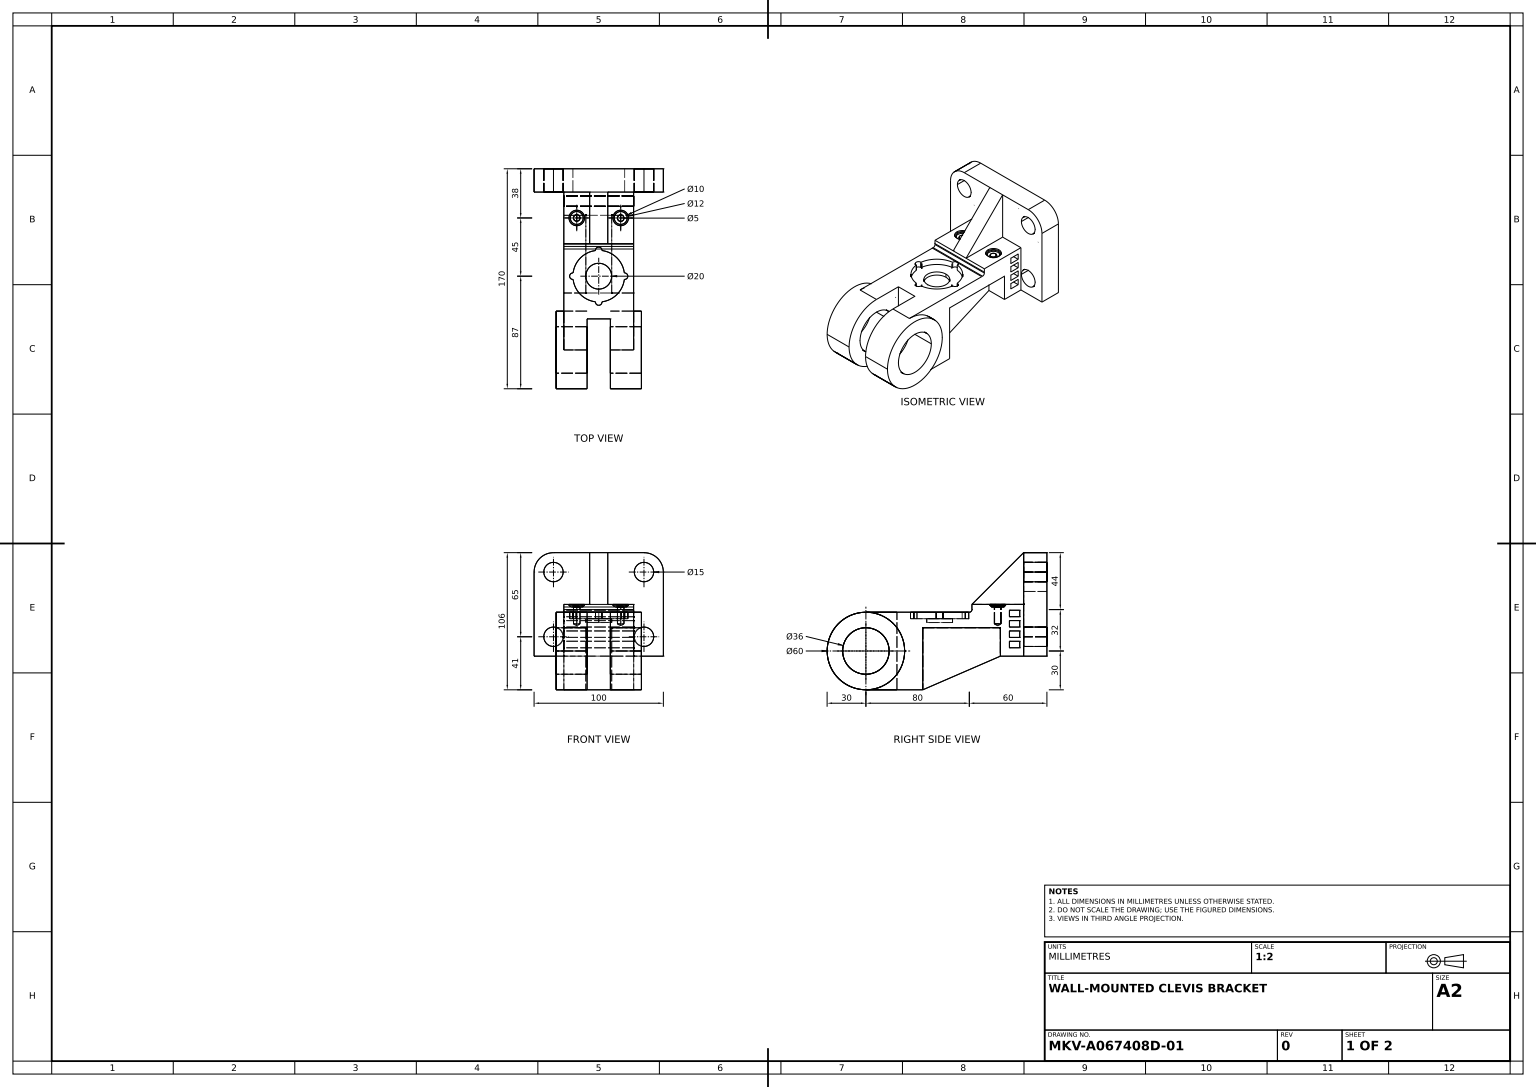
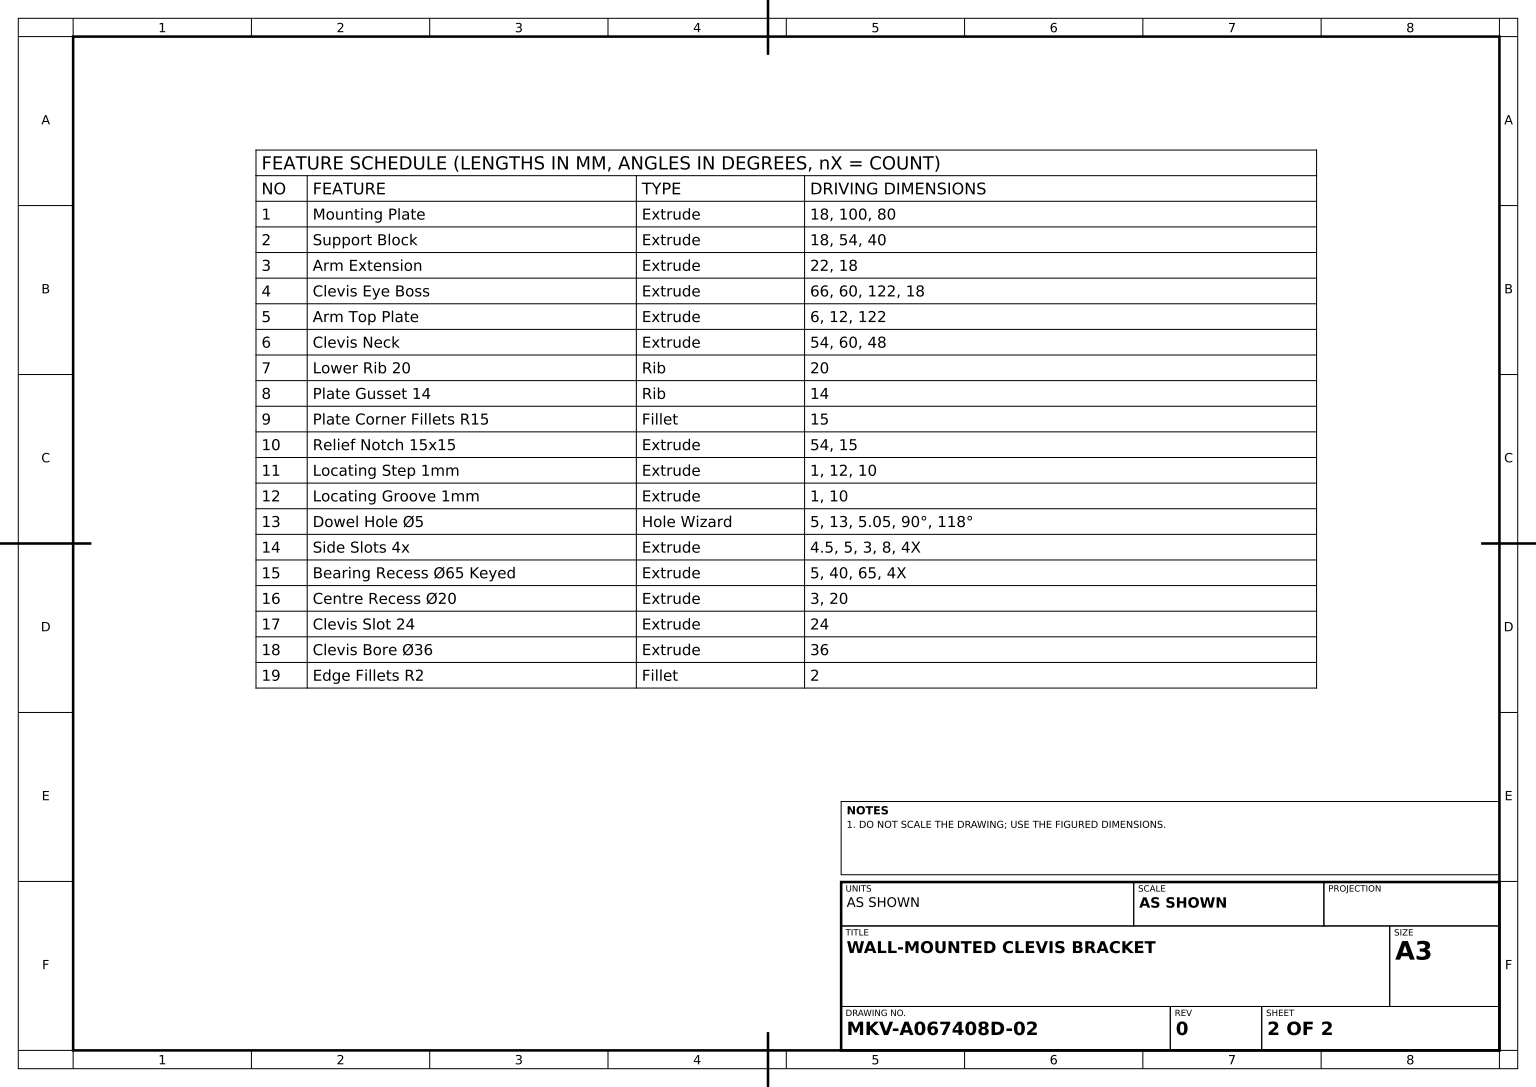
SolidWorks part; units mm, degrees
material "Plain Carbon Steel"
ref_plane "Front Plane" through (0, 0, 0) normal (0, 0, 1) x (1, 0, 0)
ref_plane "Top Plane" through (0, 0, 0) normal (0, 1, 0) x (1, 0, 0)
ref_plane "Right Plane" through (0, 0, 0) normal (1, 0, 0) x (0, 0, -1)
sketch "Mounting Plate Sketch" plane through (0, 0, 0) normal (0, 0, 1) x (1, 0, 0)
  line L1 (-50, -40) -> (50, -40)
  line L2 (-50, -40) -> (-50, 40)
  line L3 (-50, 40) -> (50, 40)
  line L4 (50, -40) -> (50, 40)
  line L5 (-50, -40) -> (50, 40) construction
  line L6 (-50, 40) -> (50, -40) construction
  point P0 (0, 0)
  dimension "D1" = 100
  dimension "D2" = 80
extrude "Mounting Plate" add sketch "Mounting Plate Sketch" along normal blind 18
sketch "Support Block Sketch" plane through (0, 0, 18) normal (0, 0, 1) x (1, 0, 0)
  line L0 (-50, -40) -> (50, -40) construction
  line L1 (-27, -40) -> (27, -40)
  line L2 (-27, -40) -> (-27, 0)
  line L3 (-27, 0) -> (27, 0)
  line L4 (27, -40) -> (27, 0)
  line L5 (0, 0) -> (0, -10.9792) construction
  dimension "D1" = 54
  dimension "D2" = 40
extrude "Support Block" add sketch "Support Block Sketch" along normal blind 18
sketch "Arm Extension Sketch" plane through (0, 0, 36) normal (0, 0, 1) x (1, 0, 0)
  line L0 (27, -40) -> (27, 0) construction
  line L1 (-27, 0) -> (27, 0)
  line L2 (-27, 0) -> (-27, -18)
  line L3 (-27, -18) -> (27, -18)
  line L4 (27, 0) -> (27, -18)
  dimension "D1" = 18
extrude "Arm Extension" add sketch "Arm Extension Sketch" along normal blind 22
sketch "Clevis Eye Sketch" plane through (0, 0, 0) normal (1, 0, 0) x (0, 0, -1)
  line L0 (-18, 40) -> (-18, -40) construction
  line L4 (-58, -18) -> (-36, -18) construction
  circle A0 centre (-140, -36) radius 30
  dimension "D1" = 60
  dimension "D2" = 122
  dimension "D3" = 18
extrude "Clevis Eye Boss" add sketch "Clevis Eye Sketch" along normal mid plane 66 separate body
ref_plane "Plane2" through (0, -6, 0) normal (0, 1, 0) x (1, 0, 0)
sketch "Arm Top Plate Sketch" plane through (0, -6, 0) normal (0, 1, 0) x (1, 0, 0)
  line L0 (33, -170) -> (33, -110) construction
  line L1 (-27, -58) -> (27, -58)
  line L2 (-27, -58) -> (-27, -140)
  line L3 (-27, -140) -> (27, -140)
  line L4 (27, -58) -> (27, -140)
  line L5 (50, -18) -> (-50, -18) construction
  dimension "D1" = 6
  dimension "D2" = 122
extrude "Arm Top Plate" add sketch "Arm Top Plate Sketch" against normal blind 12
sketch "Clevis Neck Sketch" plane through (-27, 0, 0) normal (-1, 0, 0) x (0, 0, 1)
  line L0 (116, -18) -> (36, -18) construction
  line L1 (96, -18) -> (140, -18)
  line L2 (96, -18) -> (96, -66)
  line L3 (96, -66) -> (140, -66)
  line L4 (140, -18) -> (140, -66)
  line L5 (36, -18) -> (36, -40) construction
  circle A0 centre (140, -36) radius 30 construction
  dimension "D1" = 60
  dimension "D2" = 48
extrude "Clevis Neck" add sketch "Clevis Neck Sketch" against normal blind 54
sketch "Lower Rib Sketch" plane through (0, 0, 0) normal (1, 0, 0) x (0, 0, -1)
  line L0 (-36, -40) -> (-96, -66)
rib "Lower Rib 20" sketch "Lower Rib Sketch" sketch "Lower Rib Sketch" thickness 20 extrusion direction parallel to sketch draft on no parameters "D1"=20
sketch "Plate Gusset Sketch" plane through (0, 0, 0) normal (1, 0, 0) x (0, 0, -1)
  line L0 (-18, 40) -> (-58, 0)
rib "Plate Gusset 14" sketch "Plate Gusset Sketch" sketch "Plate Gusset Sketch" thickness 14 extrusion direction parallel to sketch draft on no parameters "D1"=14
fillet "Plate Corner Fillets R15" radius 15 2 edges at (-50, 40, 9) (50, 40, 9)
sketch "Relief Notch Sketch" plane through (0, 0, 18) normal (0, 0, 1) x (1, 0, 0)
  line L0 (-50, -40) -> (-27, -40) construction
  circle A0 centre (-35, 25) radius 7.5
  circle A1 centre (-35, -25) radius 7.5
  circle A2 centre (35, 25) radius 7.5
  circle A3 centre (35, -25) radius 7.5
  dimension "D1" = 15
  dimension "D2" = 15
extrude "Relief Notch 15x15" cut sketch "Relief Notch Sketch" against normal blind 54
sketch "Locating Step Sketch" plane through (0, 0, 0) normal (0, 1, 0) x (1, 0, 0)
  line L0 (-7, -18) -> (-7, -58) construction
  line L2 (-27, -58) -> (-27, -18) construction
  line L3 (7, -18) -> (7, -58) construction
  circle A0 centre (-17, -38) radius 6
  circle A1 centre (17, -38) radius 6
  point P8 (-27, -38)
  dimension "D1" = 12
  dimension "D3" = 10
  dimension "D2" = 10
extrude "Locating Step 1mm" cut sketch "Locating Step Sketch" against normal blind 1
sketch "Locating Groove Sketch" plane through (0, -1, 0) normal (0, 1, 0) x (1, 0, 0)
  circle A0 centre (-17, -38) radius 5
  circle A1 centre (17, -38) radius 5
  dimension "D1" = 10
extrude "Locating Groove 1mm" cut sketch "Locating Groove Sketch" against normal blind 1
hole_wizard "Dowel Hole Ø5" positions "Sketch15" profile "Sketch16" hole size "Ø5.0" standard "ISO"
sketch "Sketch15" plane through (0, -2, 0) normal (0, 1, 0) x (1, 0, 0)
  point P0 (-17, -38)
  point P3 (17, -38.1219)
sketch "Sketch16" plane through (-17, -2, 38) normal (1, 0, 0) x (0, 0, 1)
  line L0 (0, 0) -> (0, 14.5022)
  line L1 (0, 14.5022) -> (2.5, 13)
  line L2 (2.5, 13) -> (2.5, 0.025)
  line L3 (2.5, 0.025) -> (2.525, 0)
  line L5 (2.525, 0) -> (0, 0)
  line L6 (-2.5, 0.025) -> (-2.525, 0) construction
  line L10 (0, 14.5022) -> (-2.5, 13) construction
  line L11 (0, -6.35) -> (0, 107.95) construction
  dimension "Hole Dia." = 5
  dimension "Hole Depth" = 13
  dimension "Near C'Sink Dia." = 5.05
  dimension "Near C'Sink Angle" = 90
  dimension "Drill Angle" = 118
sketch "Side Slots Sketch" plane through (-27, 0, 0) normal (-1, 0, 0) x (0, 0, 1)
  line L0 (58, 0) -> (18, 0) construction
  line L1 (21, -4.5) -> (29, -4.5)
  line L2 (21, -4.5) -> (21, -9.5)
  line L3 (21, -9.5) -> (29, -9.5)
  line L4 (29, -4.5) -> (29, -9.5)
  line L5 (18, 25) -> (18, -40) construction
  line L6 (21, -12.5) -> (29, -12.5)
  line L7 (21, -12.5) -> (21, -17.5)
  line L8 (21, -17.5) -> (29, -17.5)
  line L9 (29, -12.5) -> (29, -17.5)
  line L10 (21, -20.5) -> (29, -20.5)
  line L11 (21, -20.5) -> (21, -25.5)
  line L12 (21, -25.5) -> (29, -25.5)
  line L13 (29, -20.5) -> (29, -25.5)
  line L14 (21, -28.5) -> (29, -28.5)
  line L15 (21, -28.5) -> (21, -33.5)
  line L16 (21, -33.5) -> (29, -33.5)
  line L17 (29, -28.5) -> (29, -33.5)
  dimension "D1" = 4.5
  dimension "D2" = 5
  dimension "D3" = 3
  dimension "D4" = 8
  dimension "D6" = 3
  dimension "D5" = 4
extrude "Side Slots 4x" cut sketch "Side Slots Sketch" against normal through all
sketch "Bearing Recess Sketch" plane through (0, -6, 0) normal (0, 1, 0) x (1, 0, 0)
  line L0 (35, -18) -> (7, -18) construction
  arc A0 (-19.8437, -85.4951) -> (-2.4951, -102.8438) centre (0, -83) ccw
  arc A1 (2.4951, -63.1562) -> (-2.4951, -63.1562) centre (0, -63) ccw
  arc A2 (19.8438, -85.4951) -> (19.8437, -80.5049) centre (20, -83) ccw
  arc A3 (-2.4951, -102.8438) -> (2.4951, -102.8438) centre (0, -103) ccw
  arc A4 (-19.8438, -80.5049) -> (-19.8437, -85.4951) centre (-20, -83) ccw
  arc A5 (-2.4951, -63.1562) -> (-19.8438, -80.5049) centre (0, -83) ccw
  arc A6 (19.8437, -80.5049) -> (2.4951, -63.1562) centre (0, -83) ccw
  arc A7 (2.4951, -102.8438) -> (19.8438, -85.4951) centre (0, -83) ccw
  dimension "D1" = 40
  dimension "D3" = 5
  dimension "D2" = 65
  dimension "D4" = 4
extrude "Bearing Recess Ø65 Keyed" cut sketch "Bearing Recess Sketch" against normal blind 5
sketch "Centre Recess Sketch" plane through (0, -11, 0) normal (0, 1, 0) x (1, 0, 0)
  circle A0 centre (0, -83) radius 10
  dimension "D1" = 20
extrude "Centre Recess Ø20" cut sketch "Centre Recess Sketch" against normal blind 3
sketch "Clevis Slot Sketch" plane through (0, -6, 0) normal (0, 1, 0) x (1, 0, 0)
  line L0 (-27, -140) -> (27, -140) construction
  line L1 (-9, -116) -> (9, -116)
  line L2 (-9, -116) -> (-9, -189.377)
  line L3 (-9, -189.377) -> (9, -189.377)
  line L4 (9, -116) -> (9, -189.377)
  point P4 (0, -116)
  dimension "D1" = 10.8438
  dimension "D2" = 24
  dimension "D3" = 108.8721
extrude "Clevis Slot 24" cut sketch "Clevis Slot Sketch" against normal through all
sketch "Clevis Bore Sketch" plane through (-33, 0, 0) normal (-1, 0, 0) x (0, 0, 1)
  circle A0 centre (140, -36) radius 18
  dimension "D1" = 36
extrude "Clevis Bore Ø36" cut sketch "Clevis Bore Sketch" against normal through all
fillet "Edge Fillets R2" radius 2 1 edges at (0, -6, 58)
